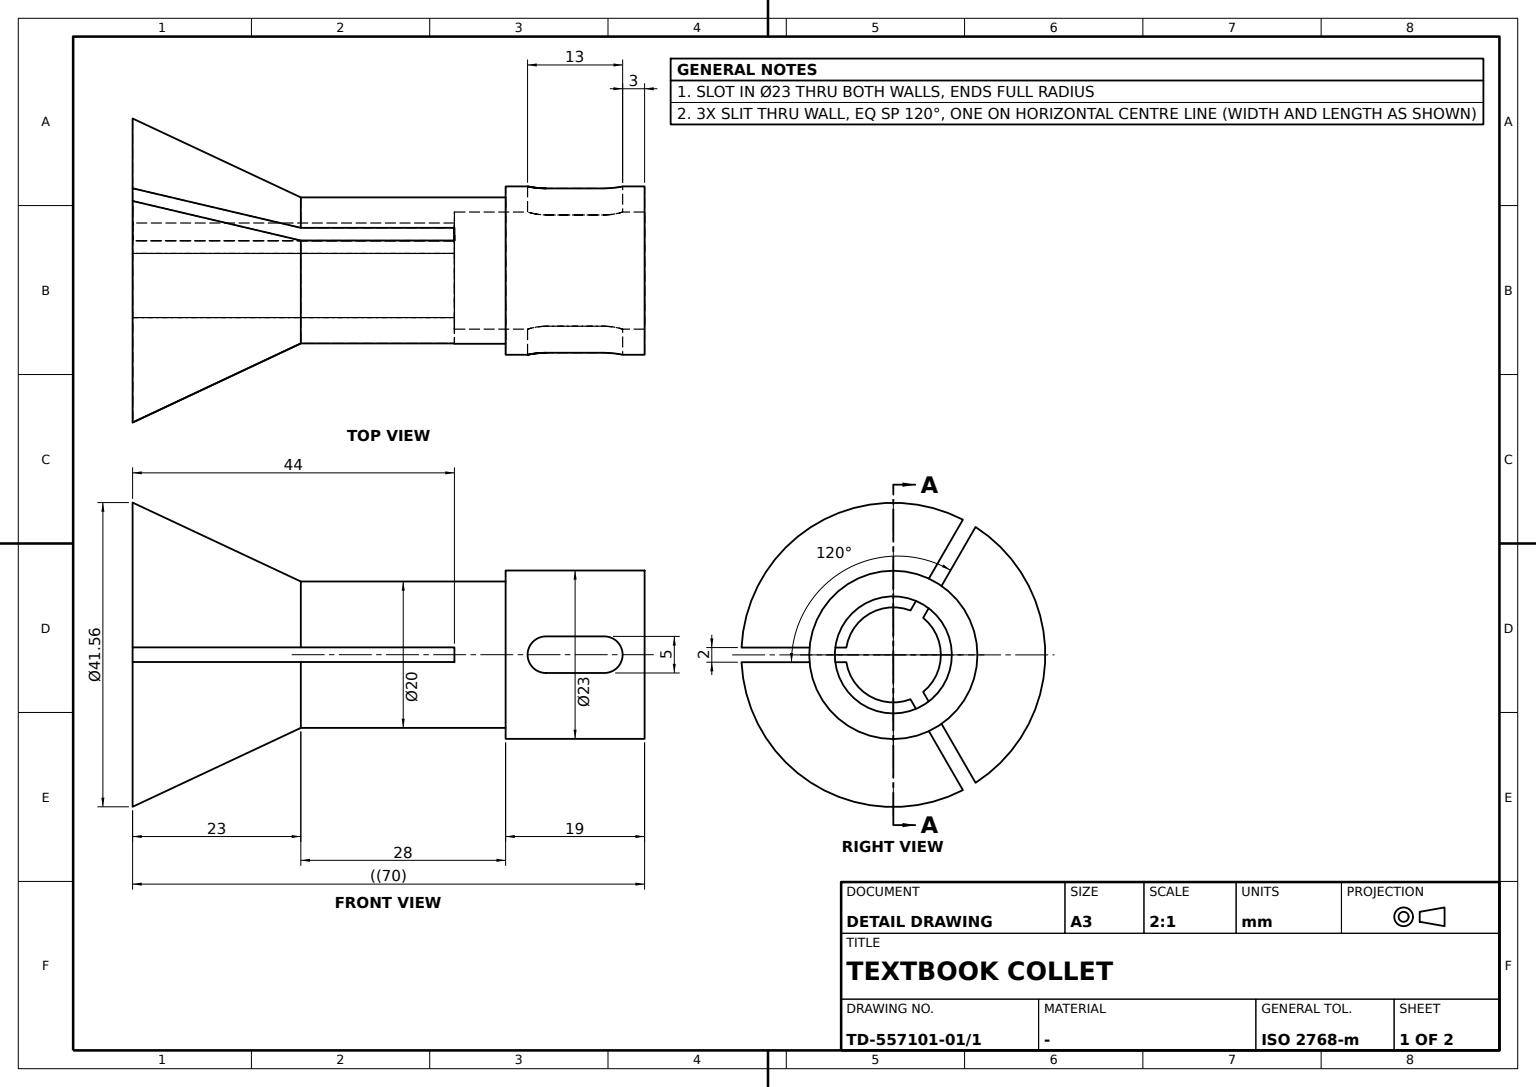
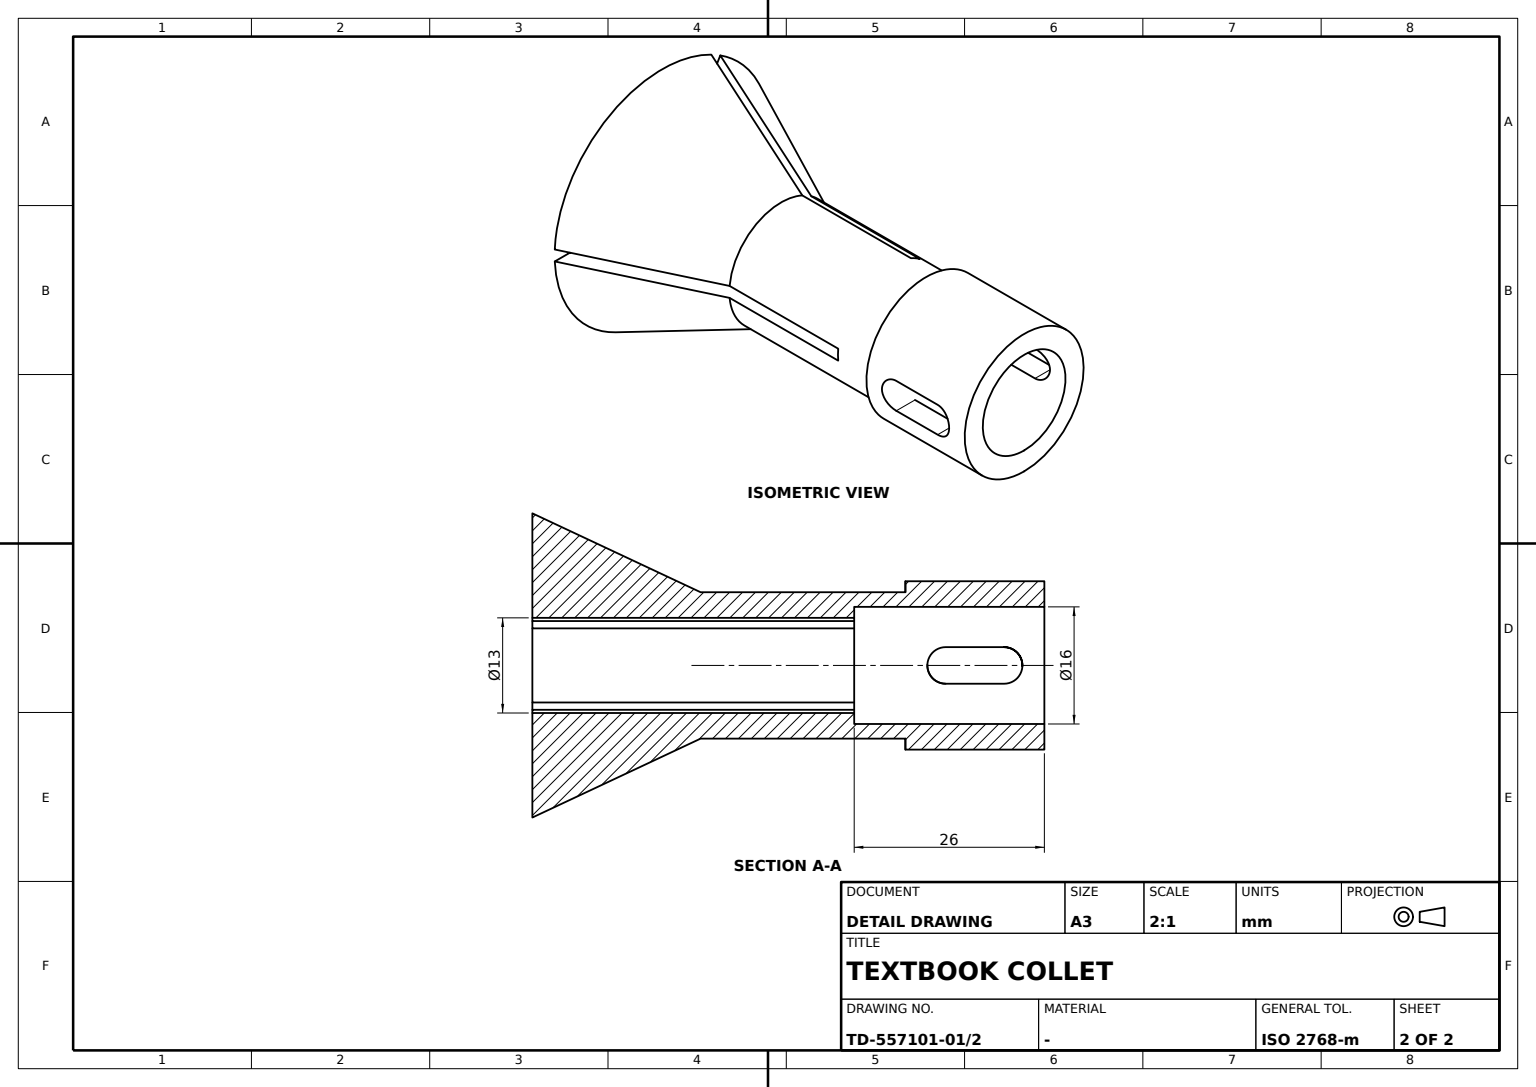
CATIA V5 part; units mm, degrees
sketch "Sketch1" plane through (0, 0, 0) normal (0, 1, 0) x (-1, 0, 0)
  line L0 (0, 0) -> (0, 11.5)
  line L1 (0, 11.5) -> (19, 11.5)
  line L2 (19, 11.5) -> (19, 10)
  line L3 (19, 10) -> (47, 10)
  line L4 (47, 10) -> (70, 20.78)
  line L5 (70, 20.78) -> (70, 0)
  point P0 (70, 0)
  line L6 (70, 0) -> (0, 0)
  point P1 (0, 0)
  dimension "length L1" = 19
  dimension "length L4 x axis" = 23
  dimension "length L3" = 28
  dimension "length L5" = 20.78
  dimension "distance L3 L6" = 10
  dimension "distance L1 L6" = 11.5
  constraint vertical L0 y-axis
  constraint vertical L2 y-axis
  constraint vertical L5 y-axis
  constraint horizontal L1 x-axis
  constraint horizontal L3 x-axis
  constraint horizontal L6 x-axis
  constraint coincidence P0 x-axis
  constraint coincidence origin L6
  constraint coincidence origin P1
revolve "Shaft1" add sketch "Sketch1" angle 360 about axis through (0, 0, 0) along (1, 0, 0)
sketch "Sketch2" plane through (-70, 0, 0) normal (-1, 0, 0) x (0, -1, 0)
  circle A0 centre (0, 0) radius 6.5
  dimension "radius A0" = 6.5
extrude "Pocket1" cut sketch "Sketch2" against normal blind 44
sketch "Sketch3" plane through (0, 0, 0) normal (1, 0, 0) x (0, 0, 1)
  circle A0 centre (0, 0) radius 8
  dimension "radius A0" = 8
extrude "Pocket2" cut sketch "Sketch3" against normal blind 26
sketch "Sketch4" plane through (-70, 0, 0) normal (-1, 0, 0) x (0, 0, 1)
  point P0 (0, -13.6688)
  line L0 (1, -6.4226) -> (1, -20.7559)
  line L1 (-1, -20.7559) -> (-1, -6.4226)
  point P1 (1, -21.1528)
  point P2 (-1, -21.1528)
  circle A0 centre (0, 0) radius 6.5 construction
  arc A1 (-1, -6.4226) -> (1, -6.4226) centre (0, 0) ccw
  circle A2 centre (0, 0) radius 20.78 construction
  arc A3 (-1, -20.7559) -> (1, -20.7559) centre (0, 0) ccw
  point P3 (-1, -6.4226)
  point P4 (-1, -6.4226)
  point P5 (1, -20.7559)
  point P6 (-1, -20.7559)
  dimension "distance L0 L1" = 2
  constraint coincidence P0 y-axis
  constraint coincidence L1 P3
  constraint coincidence A0 P4
  constraint coincidence A2 P5
  constraint coincidence A2 P6
  constraint coincidence P3 P4
  constraint vertical L0 y-axis
  constraint vertical L1 y-axis
  constraint equidistance L0 L1 P0
  constraint symmetry L0 L1 y-axis
extrude "Pocket3" cut sketch "Sketch4" against normal blind 44
pattern_circular "CircPattern1" count 3 over 360 about axis through (0, 0, 0) along (1, 0, 0) of "Pocket3"
ref_plane "Plane1" through (0, -11.5, 0) normal (0, 1, 0) x (0, 0, 1)
sketch "Sketch5" plane through (0, -11.5, 0) normal (0, 1, 0) x (0, 0, 1)
  line L0 (0, -13.5) -> (0, -5.5) construction
  point P0 (0, -13.5)
  line L1 (-2.5, -13.5) -> (-2.5, -5.5)
  line L2 (2.5, -5.5) -> (2.5, -13.5)
  arc A0 (-2.5, -5.5) -> (2.5, -5.5) centre (0, -5.5) cw
  arc A1 (2.5, -13.5) -> (-2.5, -13.5) centre (0, -13.5) cw
  line L3 (-11.5, 0) -> (11.5, 0) construction
  dimension "distance L0 L1" = 2.5
  dimension "distance A0 A1" = 13
  dimension "distance A0 L3" = 3
  constraint coincidence P0 y-axis
  constraint vertical L0 y-axis
  constraint tangency A0 L1
  constraint tangency A1 L1
  constraint tangency A0 L2
  constraint tangency A1 L2
  constraint symmetry L2 L1 y-axis
extrude "Pocket4" cut sketch "Sketch5" along normal through all
equation "\"angular step@CircPattern1\" = 360.0*1 deg/CircPattern1.AngularNumber"
